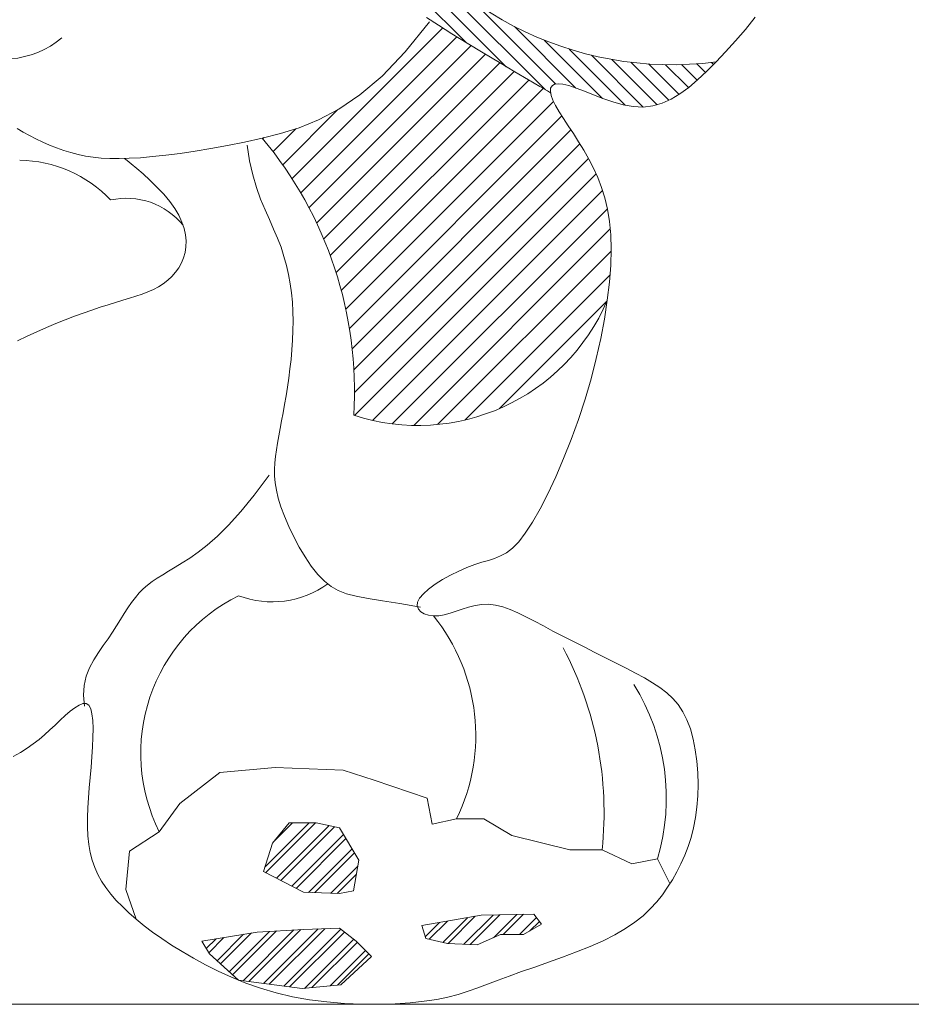
# Model space of a CAD drawing. Units: inches. Extents: x -17 to 1735, y -531 to 60.
# Tile 9 of 27: x 1734.675388 to 1734.679153, y -150.224179 to -150.220021. Entities that reach past the tile are written whole.
import ezdxf

# ---------------------------------------------------------------- set-up
doc = ezdxf.new("R2010")
doc.units = ezdxf.units.IN
doc.header["$MEASUREMENT"] = 0
doc.layers.add('A-FURN', color=242, linetype='Continuous', lineweight=18, true_color=0xcd2027)

# ---------------------------------------------------------------- blocks, each defined once
blk = doc.blocks.new('childrens_room_2')
for p, q in [((70.23120320653427, 54.05747840204134), (70.20236759360299, 54.08631401495807)), ((70.22698188498501, 54.05997091540342), (70.20319665329183, 54.0837561470675)), ((70.22263468104532, 54.06258931114138), (70.2050974529225, 54.08012653924237)), ((70.23229530256825, 54.0581151142091), (70.22340834805394, 54.06700206872341)), ((70.21842630278437, 54.06525539631406), (70.2196992340719, 54.06442092767832)), ((70.25366742467625, 54.06526988009722), (70.25262300519854, 54.06396623705081)), ((70.20400690125419, 54.04797145385822), (70.22016325000325, 54.06412780261456)), ((70.21614516905859, 54.06155212750167), (70.21875777329436, 54.06477708416645)), ((70.2196992340719, 54.06442092767832), (70.22114598193323, 54.06350699770559)), ((70.23445100571146, 54.05768821923851), (70.22784723080579, 54.06429199416601)), ((70.20494434069727, 54.04643916731441), (70.22168184573414, 54.06317667238039)), ((70.22114598193323, 54.06350699770559), (70.22277310794335, 54.06250397992557)), ((70.25262300519854, 54.06396623705081), (70.2515651093668, 54.06273375425229)), ((70.2058254618419, 54.04485056245033), (70.22321238294128, 54.06223748356428)), ((70.22277310794335, 54.06250397992557), (70.22450529499795, 54.06145310850701)), ((70.23729513219908, 54.05657290098173), (70.2310376150522, 54.06283041811406)), ((70.2515651093668, 54.06273375425229), (70.25051106391359, 54.06157435496282)), ((70.2066481458128, 54.04320352047074), (70.22475057818112, 54.06130595283906)), ((70.21366017778521, 54.05897447190222), (70.21614516905859, 54.06155212750167)), ((70.22450529499795, 54.06145310850701), (70.22624675651198, 54.06040833276205)), ((70.23974478501944, 54.05585205634128), (70.23372672202416, 54.06187011934384)), ((70.24167690089556, 54.05564874865962), (70.23611844704602, 54.06120720250914)), ((70.25051106391359, 54.06157435496282), (70.24947819562979, 54.06048996242901)), ((70.20740978735151, 54.04149543597163), (70.22629435937736, 54.06038000802658)), ((70.22624675651198, 54.06040833276205), (70.22790170590045, 54.05942360201009)), ((70.24315860012896, 54.0558958576425), (70.23830463429798, 54.06074982344438)), ((70.24441215903383, 54.05637110691754), (70.24033614836983, 54.06044711760336)), ((70.24551432266483, 54.05699775149554), (70.24224470166838, 54.06026737249925)), ((70.24651573046461, 54.05772515188295), (70.24405166280806, 54.06018921954677)), ((70.24745069189115, 54.05851899867997), (70.24577224395355, 54.06019744662484)), ((70.24834285863793, 54.05935564009855), (70.24741772615701, 54.06028077257946)), ((70.24947819562979, 54.06048996242901), (70.24847917870969, 54.05948426287654)), ((70.24920867151698, 54.0602186354285), (70.24899674283691, 54.06043056410857)), ((70.20810719999602, 54.03972312265108), (70.22784275591724, 54.05945867853592)), ((70.21129174275441, 54.05695870166386), (70.21366017778521, 54.05897447190222)), ((70.22790170590045, 54.05942360201009), (70.22937435646193, 54.05855286557784)), ((70.24847917870969, 54.05948426287654), (70.24750807719423, 54.05856799445468)), ((70.20873648953742, 54.03788268616921), (70.22939470015584, 54.05854089683129)), ((70.22937435646193, 54.05855286557784), (70.23056892155321, 54.05785007276285)), ((70.23056892155321, 54.05785007276285), (70.23138961453108, 54.05736917290636)), ((70.2318895930762, 54.05793588597447), (70.23174087157125, 54.05768089501947)), ((70.23215767678224, 54.05809471441756), (70.2318895930762, 54.05793588597447)), ((70.23254801054603, 54.05815257223588), (70.23215767678224, 54.05809471441756)), ((70.23306348210784, 54.05810465128019), (70.23254801054603, 54.05815257223588)), ((70.23370697932435, 54.0579461434449), (70.23306348210784, 54.05810465128019)), ((70.23447721871665, 54.05767913224412), (70.23370697932435, 54.0579461434449)), ((70.2465543024114, 54.05775365828453), (70.2456072658056, 54.05705375550173)), ((70.24750807719423, 54.05856799445468), (70.2465543024114, 54.05775365828453)), ((70.20902880730458, 54.05541940107508), (70.21129174275441, 54.05695870166386)), ((70.20929288009532, 54.03596935074023), (70.23095019063797, 54.05762666126832)), ((70.23138961453108, 54.05736917290636), (70.23174064886874, 54.05716411530597)), ((70.23174087157125, 54.05768089501947), (70.2317086245271, 54.05733454967998)), ((70.2317086245271, 54.05733454967998), (70.23178996414529, 54.05690165809068)), ((70.23178996414529, 54.05690165809068), (70.23198200256913, 54.05638702836444)), ((70.23535623175442, 54.05733326777994), (70.23447721871665, 54.05767913224412)), ((70.23632187868819, 54.05694509181052), (70.23535623175442, 54.05733326777994)), ((70.23735201976845, 54.05655114608674), (70.23632187868819, 54.05694509181052)), ((70.2456072658056, 54.05705375550173), (70.24465637882125, 54.05648078722737)), ((70.20977047372028, 54.0339772183492), (70.2320358858083, 54.05624263048088)), ((70.23198200256913, 54.05638702836444), (70.23227928510053, 54.05579578918554)), ((70.23227928510053, 54.05579578918554), (70.23266608932639, 54.05513435136384)), ((70.23842451512931, 54.05618797235951), (70.23735201976845, 54.05655114608674)), ((70.23951722507948, 54.05589211238697), (70.23842451512931, 54.05618797235951)), ((70.24060800981127, 54.05570010792001), (70.23951722507948, 54.05589211238697)), ((70.24167472957518, 54.05564850070954), (70.24060800981127, 54.05570010792001)), ((70.24270069931984, 54.05576565871019), (70.24167472957518, 54.05564850070954)), ((70.24369105284453, 54.05604725458982), (70.24270069931984, 54.05576565871019)), ((70.24465637882125, 54.05648078722737), (70.24369105284453, 54.05604725458982)), ((70.20301484620316, 54.04944912482318), (70.2089359568886, 54.05537023552319)), ((70.20686031459948, 54.05427115440983), (70.20902880730458, 54.05541940107508)), ((70.21016190813273, 54.03189892678205), (70.23294922768721, 54.05468624633653)), ((70.23266608932639, 54.05513435136384), (70.23312412575936, 54.05440944629521)), ((70.20477520797752, 54.05342854597114), (70.20686031459948, 54.05427115440983)), ((70.23312412575936, 54.05440944629521), (70.23363510520315, 54.05362780535364)), ((70.23363510520315, 54.05362780535364), (70.2341807381704, 54.05279615989861)), ((70.17451896065498, 54.0533605731602), (70.17516499910155, 54.05296905373546)), ((70.17516499910155, 54.05296905373546), (70.17584109301563, 54.05258956639449)), ((70.17584109301563, 54.05258956639449), (70.17654310266838, 54.05222553939387)), ((70.20081092616194, 54.05231858088376), (70.20276243071886, 54.05280616003295)), ((70.20196951501887, 54.05087351964761), (70.20441233455088, 54.05331633915051)), ((70.20276243071886, 54.05280616003295), (70.20477520797752, 54.05342854597114)), ((70.21045785759227, 54.02972515027653), (70.23392248806661, 54.05318978074359)), ((70.2341807381704, 54.05279615989861), (70.23474273529021, 54.05192124131867)), ((70.17654310266838, 54.05222553939387), (70.17726688838914, 54.05188040101205)), ((70.17726688838914, 54.05188040101205), (70.1780083105655, 54.05155757950564)), ((70.1780083105655, 54.05155757950564), (70.17876322946861, 54.0512605031385)), ((70.19530169218663, 54.05118995428932), (70.19707364461968, 54.05151860300105)), ((70.19707364461968, 54.05151860300105), (70.19891290449189, 54.0518944456839)), ((70.19891290449189, 54.0518944456839), (70.20081092616194, 54.05231858088376)), ((70.19944830472699, 54.04987592038963), (70.19918155060034, 54.051552788906)), ((70.20087192290114, 54.05224565353131), (70.20098945546081, 54.05236318604005)), ((70.21064627858462, 54.02744384521651), (70.23488772254089, 54.05168528922371)), ((70.23474273529021, 54.05192124131867), (70.23530280724982, 54.05100978098056)), ((70.17876322946861, 54.0512605031385), (70.17952750542784, 54.05099260018181)), ((70.17952750542784, 54.05099260018181), (70.18029699883076, 54.05075729889944)), ((70.18029699883076, 54.05075729889944), (70.18107070792351, 54.05055755143843)), ((70.18107070792351, 54.05055755143843), (70.18186018279405, 54.0503944055003)), ((70.18186018279405, 54.0503944055003), (70.18268011150533, 54.05026843268427)), ((70.18905787269935, 54.05032532816261), (70.19047513750732, 54.05047618649263)), ((70.19047513750732, 54.05047618649263), (70.19199389284361, 54.05066984459558)), ((70.19199389284361, 54.05066984459558), (70.1936055930087, 54.05090740101008)), ((70.1936055930087, 54.05090740101008), (70.19530169218663, 54.05118995428932)), ((70.23530280724982, 54.05100978098056), (70.23584266462015, 54.05006851025831)), ((70.18268011150533, 54.05026843268427), (70.1835451821203, 54.05018020457504)), ((70.1835451821203, 54.05018020457504), (70.18447008264368, 54.05013029277182)), ((70.18447008264368, 54.05013029277182), (70.18546950113844, 54.05011926885203)), ((70.18546950113844, 54.05011926885203), (70.18655812566752, 54.05014770441488)), ((70.18604057894439, 54.05013418576567), (70.1863111720991, 54.04991925461075)), ((70.1863111720991, 54.04991925461075), (70.18676120567719, 54.04955367698716)), ((70.18655812566752, 54.05014770441488), (70.18775064429386, 54.05021617104506)), ((70.18676120567719, 54.04955367698716), (70.18734889874352, 54.04906127812722)), ((70.18775064429386, 54.05021617104506), (70.18905787269935, 54.05032532816261)), ((70.1997931965266, 54.04836899507649), (70.19944830472699, 54.04987592038963)), ((70.21071122081369, 54.02503906145142), (70.23580548837666, 54.05013332902893)), ((70.23584266462015, 54.05006851025831), (70.2363459431904, 54.04910047430752)), ((70.18734889874352, 54.04906127812722), (70.18803247042118, 54.04846588327058)), ((70.18803247042118, 54.04846588327058), (70.18877013994964, 54.04779131765685)), ((70.20019748447115, 54.04700839372384), (70.1997931965266, 54.04836899507649)), ((70.21071357065696, 54.02257168532236), (70.23662629887579, 54.04848441356302)), ((70.2363459431904, 54.04910047430752), (70.23680397968158, 54.04809397335196)), ((70.18877013994964, 54.04779131765685), (70.18952012633557, 54.04706140653292)), ((70.23680397968158, 54.04809397335196), (70.23721003580025, 54.04703362138246)), ((70.18952012633557, 54.04706140653292), (70.19024064876024, 54.04629997513115)), ((70.19024064876024, 54.04629997513115), (70.19088992640494, 54.04553084869843)), ((70.2006424270908, 54.0457704971181), (70.20019748447115, 54.04700839372384)), ((70.21265150427237, 54.02203989292906), (70.2373123836692, 54.04670077231862)), ((70.23721003580025, 54.04703362138246), (70.23755737342756, 54.04590403241167)), ((70.19088992640494, 54.04553084869843), (70.19143405482058, 54.04477412162527)), ((70.20110928285752, 54.04463168603109), (70.2006424270908, 54.0457704971181)), ((70.23755737342756, 54.04590403241167), (70.23783925432829, 54.04468982043766)), ((70.19143405482058, 54.04477412162527), (70.19187063579332, 54.04403496495655)), ((70.19187063579332, 54.04403496495655), (70.1922051476536, 54.04331481888078)), ((70.20157931024326, 54.04356834124195), (70.20110928285752, 54.04463168603109)), ((70.2147521691036, 54.02167083178795), (70.23782642419567, 54.04474508685092)), ((70.23783925432829, 54.04468982043766), (70.2380489403836, 54.04337559945128)), ((70.1922051476536, 54.04331481888078), (70.19244306867361, 54.04261512360102)), ((70.20203376783641, 54.0425568435225), (70.20157931024326, 54.04356834124195)), ((70.2380489403836, 54.04337559945128), (70.23817969335826, 54.04194598346515)), ((70.19244306867361, 54.04261512360102), (70.19258987712558, 54.04193731929848)), ((70.19258987712558, 54.04193731929848), (70.19265105128173, 54.04128284617621)), ((70.2024539139343, 54.0415735736446), (70.20203376783641, 54.0425568435225)), ((70.21705303836964, 54.02150197504528), (70.23812249018695, 54.04257142684804)), ((70.23817969335826, 54.04194598346515), (70.23822477507522, 54.04038558647011)), ((70.19265105128173, 54.04128284617621), (70.19263206947247, 54.04065314442999)), ((70.2028244671051, 54.04059846488093), (70.2024539139343, 54.0415735736446)), ((70.19253840997001, 54.0400496542556), (70.1923754068662, 54.03947386384828)), ((70.19263206947247, 54.04065314442999), (70.19253840997001, 54.0400496542556)), ((70.20314398571966, 54.03962566042031), (70.2028244671051, 54.04059846488093)), ((70.2196183791489, 54.02159758981582), (70.23821973999614, 54.0401989506849)), ((70.23822477507522, 54.04038558647011), (70.23817889119849, 54.03868479222587)), ((70.1921478176478, 54.03892745344496), (70.19186025562115, 54.03841215128199)), ((70.1923754068662, 54.03947386384828), (70.1921478176478, 54.03892745344496)), ((70.20341448807042, 54.03865285595969), (70.20314398571966, 54.03962566042031)), ((70.19151733403444, 54.03792968558121), (70.19112366625225, 54.03748178460086)), ((70.19186025562115, 54.03841215128199), (70.19151733403444, 54.03792968558121)), ((70.20363799244981, 54.03767774718875), (70.20341448807042, 54.03865285595969)), ((70.23817889119849, 54.03868479222587), (70.2380425230472, 54.03685706347317)), ((70.19020254515229, 54.03669658970324), (70.18968431850547, 54.03636275226602)), ((70.19068386552274, 54.03707017656273), (70.19020254515229, 54.03669658970324)), ((70.19112366625225, 54.03748178460086), (70.19068386552274, 54.03707017656273)), ((70.20381651726669, 54.03669802978988), (70.20363799244981, 54.03767774718875)), ((70.20395208075527, 54.03571139945274), (70.20381651726669, 54.03669802978988)), ((70.22257581208717, 54.02208529677449), (70.23809855385801, 54.0376080385235)), ((70.2380425230472, 54.03685706347317), (70.23781759589795, 54.0349216327217)), ((70.18854791049264, 54.03580741270565), (70.18792838359835, 54.03557035645502)), ((70.18913283764735, 54.03606866425111), (70.18854791049264, 54.03580741270565)), ((70.18968431850547, 54.03636275226602), (70.18913283764735, 54.03606866425111)), ((70.2040467012662, 54.03471555186701), (70.20395208075527, 54.03571139945274)), ((70.18508121279186, 54.03469126083513), (70.18427138764994, 54.03444556337348)), ((70.18585067161942, 54.03491794768928), (70.18508121279186, 54.03469126083513)), ((70.18658091751743, 54.03513426512512), (70.18585067161942, 54.03491794768928)), ((70.18727310369607, 54.03534885432458), (70.18658091751743, 54.03513426512512)), ((70.18792838359835, 54.03557035645502), (70.18727310369607, 54.03534885432458)), ((70.20410239720835, 54.03370818271509), (70.2040467012662, 54.03471555186701)), ((70.22626748833457, 54.02330724702773), (70.2377693360427, 54.03480909471404)), ((70.23781759589795, 54.0349216327217), (70.23750603485271, 54.03289773246655)), ((70.18161153590657, 54.03354947326301), (70.18066071702518, 54.03319816138395)), ((70.18253294507625, 54.03387486160358), (70.18161153590657, 54.03354947326301)), ((70.18342090783293, 54.034173750339), (70.18253294507625, 54.03387486160358)), ((70.18427138764994, 54.03444556337348), (70.18342090783293, 54.034173750339)), ((70.20412142703893, 54.03268823586262), (70.20410239720835, 54.03370818271509)), ((70.17868699658314, 54.03242007136435), (70.17767216825044, 54.03199444538626)), ((70.17968452507515, 54.0328215020549), (70.17868699658314, 54.03242007136435)), ((70.18066071702518, 54.03319816138395), (70.17968452507515, 54.0328215020549)), ((70.20410701051472, 54.03165964784278), (70.20412142703893, 54.03268823586262)), ((70.23750603485271, 54.03289773246655), (70.23710976507166, 54.0308045952101)), ((70.17664407677833, 54.03154520020911), (70.17560685473612, 54.03107358400887)), ((70.17767216825044, 54.03199444538626), (70.17664407677833, 54.03154520020911)), ((70.2040626076155, 54.03062760335746), (70.20410701051472, 54.03165964784278)), ((70.17560685473612, 54.03107358400887), (70.17456501944574, 54.03058353331147)), ((70.20399167832105, 54.02959728711579), (70.2040626076155, 54.03062760335746)), ((70.23710976507166, 54.0308045952101), (70.2366307118896, 54.02866145344745)), ((70.20389768249473, 54.02857388381239), (70.20399167832105, 54.02959728711579)), ((70.20378408023274, 54.02756257816367), (70.20389768249473, 54.02857388381239)), ((70.2366307118896, 54.02866145344745), (70.2360708004085, 54.02648753968827)), ((70.20365433139843, 54.02656855487151), (70.20378408023274, 54.02756257816367)), ((70.20351189597162, 54.02559699863053), (70.20365433139843, 54.02656855487151)), ((70.2360708004085, 54.02648753968827), (70.23543195578851, 54.02430208643494)), ((70.20336023393205, 54.02465232605613), (70.20351189597162, 54.02559699863053)), ((70.2032028052595, 54.02373588132326), (70.20336023393205, 54.02465232605613)), ((70.23543195578851, 54.02430208643494), (70.23471867026413, 54.022126730239)), ((70.20304306993378, 54.02284824050588), (70.2032028052595, 54.02373588132326)), ((70.20273051918369, 54.02116167492789), (70.20288448787645, 54.02198997967793)), ((70.20288448787645, 54.02198997967793), (70.20304306993378, 54.02284824050588)), ((70.23471867026413, 54.022126730239), (70.23394570355188, 54.01999272392862)), ((70.20258462371888, 54.02036390232246), (70.20273051918369, 54.02116167492789)), ((70.20245026152, 54.01959723794283), (70.20258462371888, 54.02036390232246)), ((70.23394570355188, 54.01999272392862), (70.23313038255904, 54.0179337243739)), ((70.20223093784765, 54.01815675377878), (70.20233089256683, 54.01886225786296)), ((70.20233089256683, 54.01886225786296), (70.20245026152, 54.01959723794283)), ((70.2021586629667, 54.01746737988872), (70.20223093784765, 54.01815675377878)), ((70.23313038255904, 54.0179337243739), (70.23229003396003, 54.01598338845218)), ((70.2021232944203, 54.01677800598412), (70.2021586629667, 54.01746737988872)), ((70.20213405882126, 54.01607250187812), (70.2021232944203, 54.01677800598412)), ((70.20154355682783, 54.01615852959224), (70.1999571128504, 54.01402910353358)), ((70.20220018278226, 54.01533473737657), (70.20213405882126, 54.01607250187812)), ((70.23229003396003, 54.01598338845218), (70.23144198466208, 54.01417537304809)), ((70.20233089279967, 54.01454858228539), (70.20220018278226, 54.01533473737657)), ((70.20253541554442, 54.01369790641769), (70.20233089279967, 54.01454858228539)), ((70.1999571128504, 54.01402910353358), (70.19851223927574, 54.01225771024332)), ((70.20282297745464, 54.01276657957208), (70.20253541554442, 54.01369790641769)), ((70.23144198466208, 54.01417537304809), (70.23060356128147, 54.01254333503169)), ((70.20319939335926, 54.0117468727098), (70.20282297745464, 54.01276657957208)), ((70.23060356128147, 54.01254333503169), (70.2297920907254, 54.01112093128034)), ((70.19851223927574, 54.01225771024332), (70.19719826786196, 54.01080143188886)), ((70.20365683019511, 54.01066466134802), (70.20319939335926, 54.0117468727098)), ((70.19719826786196, 54.01080143188886), (70.19600453036722, 54.00961735061577)), ((70.20418404311523, 54.00955422214469), (70.20365683019511, 54.01066466134802)), ((70.2297920907254, 54.01112093128034), (70.22902489972651, 54.00994181867139)), ((70.19600453036722, 54.00961735061577), (70.19492035854958, 54.00866254856959)), ((70.20476978715627, 54.00844983177961), (70.20418404311523, 54.00955422214469)), ((70.22902489972651, 54.00994181867139), (70.2283135394787, 54.00902651187647)), ((70.19492035854958, 54.00866254856959), (70.19393508422537, 54.0078941079177)), ((70.20540281741299, 54.0073857669035), (70.20476978715627, 54.00844983177961)), ((70.22764645878809, 54.00834295672979), (70.22700633086382, 54.0078459568453)), ((70.2283135394787, 54.00902651187647), (70.22764645878809, 54.00834295672979)), ((70.19303803903634, 54.0072691107984), (70.19221855485696, 54.00674463937178)), ((70.19393508422537, 54.0078941079177), (70.19303803903634, 54.0072691107984)), ((70.20607188909663, 54.00639630419613), (70.20540281741299, 54.0073857669035)), ((70.22573762620917, 54.00723083736233), (70.22507439589711, 54.00702232500629)), ((70.22637582891505, 54.00749031585149), (70.22573762620917, 54.00723083736233)), ((70.22700633086382, 54.0078459568453), (70.22637582891505, 54.00749031585149)), ((70.19146682841122, 54.00628267245924), (70.19077651640285, 54.00586477554174)), ((70.19221855485696, 54.00674463937178), (70.19146682841122, 54.00628267245924)), ((70.20676575718565, 54.00551572031549), (70.20607188909663, 54.00639630419613)), ((70.22276993510198, 54.00626071799928), (70.2218939703994, 54.0058747858115)), ((70.22360354546575, 54.00657741317122), (70.22276993510198, 54.00626071799928)), ((70.22436881124625, 54.0068195824046), (70.22360354546575, 54.00657741317122)), ((70.22507439589711, 54.00702232500629), (70.22436881124625, 54.0068195824046)), ((70.18955822255114, 54.00510704034099), (70.18901928416338, 54.00474012637864)), ((70.19014214055963, 54.00547741078338), (70.18955822255114, 54.00510704034099)), ((70.19077651640285, 54.00586477554174), (70.19014214055963, 54.00547741078338)), ((70.20747317694943, 54.00477829193409), (70.20676575718565, 54.00551572031549)), ((70.22015359207172, 54.00495675443238), (70.2193584855518, 54.00445542723758)), ((70.2210103048815, 54.0054350026316), (70.22015359207172, 54.00495675443238)), ((70.2218939703994, 54.0058747858115), (70.2210103048815, 54.0054350026316)), ((70.18805443304475, 54.00396251648493), (70.18761756371126, 54.00352474488176)), ((70.18851984712413, 54.00436313103859), (70.18805443304475, 54.00396251648493)), ((70.18901928416338, 54.00474012637864), (70.18851984712413, 54.00436313103859)), ((70.20819366770914, 54.00420629407602), (70.20747317694943, 54.00477829193409)), ((70.20896980627325, 54.00377399522989), (70.20819366770914, 54.00420629407602)), ((70.21865963890335, 54.00394640703456), (70.21809170570808, 54.00344507981793)), ((70.2193584855518, 54.00445542723758), (70.21865963890335, 54.00394640703456)), ((70.1872033283685, 54.00303930279045), (70.18680408615504, 54.00250777441982)), ((70.18761756371126, 54.00352474488176), (70.1872033283685, 54.00303930279045)), ((70.20985493390938, 54.00344366225039), (70.20896980627325, 54.00377399522989)), ((70.21090239171056, 54.00317756199223), (70.20985493390938, 54.00344366225039)), ((70.21216552094441, 54.00293796131013), (70.21090239171056, 54.00317756199223)), ((70.21369766264573, 54.0026871270515), (70.21216552094441, 54.00293796131013)), ((70.21768933943125, 54.00296683160417), (70.21747772815753, 54.00252560594385)), ((70.21809170570808, 54.00344507981793), (70.21768933943125, 54.00296683160417)), ((70.18641176390113, 54.00193476841235), (70.18601828837885, 54.00132489338142)), ((70.18680408615504, 54.00250777441982), (70.18641176390113, 54.00193476841235)), ((70.21555215808215, 54.00238732607107), (70.21369766264573, 54.0026871270515)), ((70.21778234846307, 54.00200082521627), (70.21555215808215, 54.00238732607107)), ((70.21747772815753, 54.00252560594385), (70.21744419763446, 54.00212957664774)), ((70.21744419763446, 54.00212957664774), (70.21756660805434, 54.00178547510444)), ((70.21756660805434, 54.00178547510444), (70.21782281972585, 54.00150003268066)), ((70.22159829189653, 54.00156269820439), (70.22225847410621, 54.00178723761786)), ((70.22225847410621, 54.00178723761786), (70.22293790826691, 54.0020002375299)), ((70.22293790826691, 54.0020002375299), (70.22363563185675, 54.00217573407139)), ((70.22363563185675, 54.00217573407139), (70.22435068217922, 54.0022877633732)), ((70.22435068217922, 54.0022877633732), (70.22508209665423, 54.00231036155168)), ((70.22508209665423, 54.00231036155168), (70.22583003581852, 54.00222397556212)), ((70.22583003581852, 54.00222397556212), (70.2265991521522, 54.00203469570846)), ((70.2265991521522, 54.00203469570846), (70.22739522119403, 54.00175502309725)), ((70.18601828837885, 54.00132489338142), (70.18561558624381, 54.00068275794769)), ((70.21782281972585, 54.00150003268066), (70.21819069284132, 54.00127998075771)), ((70.21819069284132, 54.00127998075771), (70.21864808759302, 54.00113205071687)), ((70.21864808759302, 54.00113205071687), (70.21917286423152, 54.00106297392489)), ((70.21917286423152, 54.00106297392489), (70.21974288306549, 54.00107948177032)), ((70.21974288306549, 54.00107948177032), (70.22033953376697, 54.00118285640786)), ((70.22033953376697, 54.00118285640786), (70.22095832421795, 54.00135258318044)), ((70.22095832421795, 54.00135258318044), (70.22159829189653, 54.00156269820439)), ((70.22739522119403, 54.00175502309725), (70.22822401859915, 54.00139745887139)), ((70.22822401859915, 54.00139745887139), (70.22909131996451, 54.00097450413745)), ((70.22909131996451, 54.00097450413745), (70.23000290082885, 54.00049866003104)), ((70.18519558420988, 54.00001297075363), (70.1847502091073, 53.99932014041991)), ((70.18561558624381, 54.00068275794769), (70.18519558420988, 54.00001297075363)), ((70.23000290082885, 54.00049866003104), (70.23096453684732, 53.99998242766599)), ((70.23096453684732, 53.99998242766599), (70.23198200350046, 53.99943830817796)), ((70.18427138764994, 53.99860887556719), (70.18375787035214, 53.9978810004381)), ((70.1847502091073, 53.99932014041991), (70.18427138764994, 53.99860887556719)), ((70.23198200350046, 53.99943830817796), (70.23305722606486, 53.99887752051876)), ((70.23305722606486, 53.99887752051876), (70.23417672818644, 53.99830615498507)), ((70.18375787035214, 53.9978810004381), (70.18323570316309, 53.99712720178508)), ((70.23417672818644, 53.99830615498507), (70.23532318295796, 53.99772901968976)), ((70.23532318295796, 53.99772901968976), (70.23647926376319, 53.99715092276022)), ((70.18323570316309, 53.99712720178508), (70.1827377558325, 53.99633538195343)), ((70.23647926376319, 53.99715092276022), (70.23762764375309, 53.99657667232389)), ((70.23762764375309, 53.99657667232389), (70.23875099625323, 53.99601107650818)), ((70.18229689793546, 53.99549344331029), (70.18194599927986, 53.99458928820826)), ((70.1827377558325, 53.99633538195343), (70.18229689793546, 53.99549344331029)), ((70.23875099625323, 53.99601107650818), (70.23983199435636, 53.99545894343322)), ((70.23983199435636, 53.99545894343322), (70.24085331138807, 53.99492508121915)), ((70.18194599927986, 53.99458928820826), (70.18171792961542, 53.99361081901446)), ((70.24085331138807, 53.99492508121915), (70.24180066871807, 53.99441045150019)), ((70.24180066871807, 53.99441045150019), (70.2426719808241, 53.99390062989408)), ((70.18171792961542, 53.99361081901446), (70.18164555857541, 53.99254593807421)), ((70.2426719808241, 53.99390062989408), (70.24346821028624, 53.9933773455254)), ((70.24346821028624, 53.9933773455254), (70.24419031962636, 53.99282232753325)), ((70.18164555857541, 53.99254593807421), (70.18176175590955, 53.99138254775465)), ((70.24419031962636, 53.99282232753325), (70.244839271541, 53.9922173050349)), ((70.18116161007084, 53.99149592623001), (70.1807050173625, 53.99121192631577)), ((70.18157007278526, 53.99165299162127), (70.18116161007084, 53.99149592623001)), ((70.18192077964662, 53.99165619699346), (70.18157007278526, 53.99165299162127)), ((70.18220410450479, 53.99147861685055), (70.18192077964662, 53.99165619699346)), ((70.18241346966127, 53.99110214057731), (70.18220410450479, 53.99147861685055)), ((70.244839271541, 53.9922173050349), (70.24541602849379, 53.99154400715492)), ((70.24541602849379, 53.99154400715492), (70.24592155323947, 53.99078416302512)), ((70.17968594609877, 53.9903708249389), (70.17914271955262, 53.98986757447568)), ((70.1802099207521, 53.99082791738186), (70.17968594609877, 53.9903708249389)), ((70.1807050173625, 53.99121192631577), (70.1802099207521, 53.99082791738186)), ((70.1825544903509, 53.9905439171693), (70.18241346966127, 53.99110214057731)), ((70.18263582985267, 53.98982991049564), (70.1825544903509, 53.9905439171693)), ((70.24592155323947, 53.99078416302512), (70.2463568082417, 53.98991950177009)), ((70.17858986703098, 53.98934509149552), (70.17803364544991, 53.98882613445898)), ((70.17914271955262, 53.98986757447568), (70.17858986703098, 53.98934509149552)), ((70.18266615167843, 53.98898608444), (70.18263582985267, 53.98982991049564)), ((70.2463568082417, 53.98991950177009), (70.24672275619699, 53.98893864416317)), ((70.17746683531325, 53.98831679366271), (70.17687884800719, 53.98781899236059)), ((70.17803364544991, 53.98882613445898), (70.17746683531325, 53.98831679366271)), ((70.18265411910718, 53.98803840287877), (70.18266615167843, 53.98898608444)), ((70.24672275619699, 53.98893864416317), (70.24702035962721, 53.98785777755114)), ((70.17625909497613, 53.9873346538065), (70.17559698760627, 53.98686570126159)), ((70.17687884800719, 53.98781899236059), (70.17625909497613, 53.9873346538065)), ((70.18253764458817, 53.98593532877424), (70.18260839559255, 53.9870128297029)), ((70.18260839559255, 53.9870128297029), (70.18265411910718, 53.98803840287877)), ((70.24702035962721, 53.98785777755114), (70.24725058117068, 53.98669998094414)), ((70.17488193734201, 53.98641405797246), (70.17410335556954, 53.985981647193)), ((70.17559698760627, 53.98686570126159), (70.17488193734201, 53.98641405797246)), ((70.18245052937301, 53.98483186399102), (70.18253764458817, 53.98593532877424)), ((70.24725058117068, 53.98669998094414), (70.24741438340746, 53.98548833333774)), ((70.24741438340746, 53.98548833333774), (70.24751272891766, 53.98424591373481)), ((70.18235571345897, 53.98372519380649), (70.18245052937301, 53.98483186399102)), ((70.19625148678782, 53.98425861792787), (70.19197089150433, 53.98094796042136)), ((70.20218908805285, 53.98481039490292), (70.19625148678782, 53.98425861792787)), ((70.2095075273642, 53.98453450696109), (70.20218908805285, 53.98481039490292)), ((70.21282153560199, 53.98343095409512), (70.2095075273642, 53.98453450696109)), ((70.24751272891766, 53.98424591373481), (70.24754658039777, 53.98299580112364)), ((70.1822618601832, 53.98262525501053), (70.18235571345897, 53.98372519380649)), ((70.21848296887359, 53.98149973631229), (70.21282153560199, 53.98343095409512)), ((70.24754658039777, 53.98299580112364), (70.24751690031147, 53.98176107452167)), ((70.18217763288297, 53.98153877896987), (70.1822618601832, 53.98262525501053)), ((70.24751690031147, 53.98176107452167), (70.24742465135526, 53.98056481291718)), ((70.18211169495365, 53.98047249707309), (70.18217763288297, 53.98153877896987)), ((70.19197089150433, 53.98094796042136), (70.18976155145677, 53.97791318977255)), ((70.21903530486045, 53.97874085468941), (70.21848296887359, 53.98149973631229)), ((70.18207270984888, 53.97943314067965), (70.18211169495365, 53.98047249707309)), ((70.24742465135526, 53.98056481291718), (70.24727127737017, 53.97942544745314)), ((70.18206934084768, 53.97842744116355), (70.18207270984888, 53.97943314067965)), ((70.20111043187674, 53.97415213506469), (70.2058370959817, 53.97887879920602)), ((70.20117600478582, 53.97351850347916), (70.20653630049085, 53.97887879920602)), ((70.20191292005941, 53.97667169348136), (70.20370800910635, 53.97887879920602)), ((70.20214579854976, 53.97695802328093), (70.20406657446759, 53.97887879920602)), ((70.20234419779038, 53.97291617502782), (70.2079981585953, 53.97857013580363)), ((70.20370800910635, 53.97887879920602), (70.20660776826438, 53.97887879920602)), ((70.20660776826438, 53.97887879920602), (70.20909327636357, 53.97832702223098)), ((70.22165889602503, 53.97929263058035), (70.21903530486045, 53.97874085468941)), ((70.22455865512487, 53.97929263058035), (70.22165889602503, 53.97929263058035)), ((70.22759649729008, 53.97749935730684), (70.22455865512487, 53.97929263058035)), ((70.24727127737017, 53.97942544745314), (70.24706014747383, 53.97834281786931)), ((70.18211025140366, 53.97746212990608), (70.18206934084768, 53.97842744116355)), ((70.18976155145677, 53.97791318977255), (70.18658562622616, 53.97584402855722)), ((70.20280553413207, 53.97267830683126), (70.20857034013491, 53.97844311284865)), ((70.20397372719484, 53.9720759783799), (70.20951785509126, 53.97762010631999)), ((70.20909327636357, 53.97832702223098), (70.21116453148309, 53.97487842020786)), ((70.23381026462769, 53.97598197307383), (70.22759649729008, 53.97749935730684)), ((70.24706014747383, 53.97834281786931), (70.2467951120448, 53.97731211603098)), ((70.18220410485404, 53.97654393826673), (70.18211025140366, 53.97746212990608)), ((70.18235812063679, 53.97567735383785), (70.18220410485404, 53.97654393826673)), ((70.20094633499278, 53.97363692283255), (70.20191292005941, 53.97667169348136)), ((70.20443506347831, 53.97183811018334), (70.20978022257216, 53.97718326929174)), ((70.2467951120448, 53.97731211603098), (70.24648002146162, 53.97632853382532)), ((70.18257374276757, 53.97485788902708), (70.18235812063679, 53.97567735383785)), ((70.18658562622616, 53.97584402855722), (70.18617137522554, 53.97170570613383)), ((70.20577764442307, 53.97141016965765), (70.21044458793361, 53.97607711312452)), ((70.20645276190363, 53.97138608264362), (70.2107069553563, 53.97564027609627)), ((70.23726235785173, 53.97598197307383), (70.23381026462769, 53.97598197307383)), ((70.24043828494499, 53.97446458774942), (70.23726235785173, 53.97598197307383)), ((70.24611872610288, 53.9753872631249), (70.24571507646354, 53.97448349579502)), ((70.24648002146162, 53.97632853382532), (70.24611872610288, 53.9753872631249)), ((70.18285097118817, 53.97407881246039), (70.18257374276757, 53.97485788902708)), ((70.21116453148309, 53.97487842020786), (70.21061219741706, 53.97156776161722)), ((70.24319995911677, 53.97501636364035), (70.24043828494499, 53.97446458774942)), ((70.24454078638112, 53.97235958649111), (70.24319995911677, 53.97501636364035)), ((70.24571507646354, 53.97448349579502), (70.24527292286396, 53.97361242372284)), ((70.18318980584039, 53.97333339276378), (70.18285097118817, 53.97407881246039)), ((70.18359024684062, 53.97261489854867), (70.18318980584039, 53.97333339276378)), ((70.20522693021806, 53.97142981818473), (70.20094633499278, 53.97363692283255)), ((70.20816229040386, 53.97132508962972), (70.21105417988613, 53.97421697910471)), ((70.20883740788443, 53.97130100261569), (70.21091416939046, 53.97337776409989)), ((70.24527292286396, 53.97361242372284), (70.2447961156827, 53.97276923878092)), ((70.18405229413068, 53.9719165984556), (70.18359024684062, 53.97261489854867)), ((70.2447961156827, 53.97276923878092), (70.24428545707954, 53.97194993420129)), ((70.18457594776876, 53.97123176109602), (70.18405229413068, 53.9719165984556)), ((70.18516120763846, 53.9705536550959), (70.18457594776876, 53.97123176109602)), ((70.18617137522554, 53.97170570613383), (70.18729528867291, 53.96851837538855)), ((70.20909327636357, 53.97129187366812), (70.20522693021806, 53.97142981818473)), ((70.21061219741706, 53.97156776161722), (70.20909327636357, 53.97129187366812)), ((70.2437295563391, 53.97115370862451), (70.24311397452723, 53.97038056205059)), ((70.24428545707954, 53.97194993420129), (70.2437295563391, 53.97115370862451)), ((70.18580839475501, 53.96987651070816), (70.18516120763846, 53.9705536550959)), ((70.24311397452723, 53.97038056205059), (70.24242427259335, 53.96963049449408)), ((70.18651911332157, 53.96919840467893), (70.18580839475501, 53.96987651070816)), ((70.18729528867291, 53.96851837538855), (70.18651911332157, 53.96919840467893)), ((70.22994392040303, 53.96908476794346), (70.22428248713143, 53.96894682451097)), ((70.22561391892262, 53.96654918418647), (70.22810468899436, 53.96903995422184)), ((70.2266416014277, 53.96687766221152), (70.22882135539433, 53.96905741612721)), ((70.23077242246248, 53.96798121507749), (70.22994392040303, 53.96908476794346)), ((70.24242427259335, 53.96963049449408), (70.24164601160331, 53.96890350593316)), ((70.18813884585282, 53.96783546122463), (70.18729528867291, 53.96851837538855)), ((70.22428248713143, 53.96894682451097), (70.21793063480757, 53.967843271645)), ((70.21829280729756, 53.96663725052935), (70.2198285703885, 53.96817301360574)), ((70.21872843610939, 53.96637367486841), (70.22067479563296, 53.96832003439198)), ((70.22016199126259, 53.96603670847838), (70.22281760234503, 53.9686923195681)), ((70.22073469987257, 53.96591021263742), (70.22366382758949, 53.96883934035435)), ((70.22243152100012, 53.96583651222176), (70.22557328415454, 53.96897827537618)), ((70.2231016201072, 53.96580740685607), (70.2262899505545, 53.96899573728155)), ((70.2284121229418, 53.96687766221152), (70.23023350549514, 53.96869904475756)), ((70.22883925035015, 53.96687766221152), (70.23077242246248, 53.96798121507749)), ((70.22947324219741, 53.96723957696526), (70.2305333377549, 53.96829967250818)), ((70.24076475256473, 53.96819959638236), (70.23976605654346, 53.9675187658417)), ((70.24164601160331, 53.96890350593316), (70.24076475256473, 53.96819959638236)), ((70.18905171019608, 53.96714870055297), (70.18813884585282, 53.96783546122463)), ((70.19003580680467, 53.96645713176844), (70.18905171019608, 53.96714870055297)), ((70.19431831467548, 53.96618794181126), (70.20025591594052, 53.96715355124474)), ((70.19633598970134, 53.96373903642092), (70.1996523486555, 53.9670553954042)), ((70.19726816950018, 53.96290069472019), (70.2015953644982, 53.96722788974006)), ((70.19763630076662, 53.96256962149204), (70.20233565459378, 53.96726897534103)), ((70.19876223140048, 53.96192503059722), (70.20421021281393, 53.96737301206162)), ((70.19937939419063, 53.96184298894372), (70.2049505029677, 53.96741409766258)), ((70.20025591594052, 53.96715355124474), (70.20522693021806, 53.96742943918656)), ((70.20094217035106, 53.96163524355364), (70.20679221210187, 53.96748528528991)), ((70.2015593331412, 53.96155320190013), (70.20751728572534, 53.96751115444789)), ((70.20312210930163, 53.96134545650278), (70.20923507203, 53.9674584192457)), ((70.20373927209178, 53.96126341484927), (70.20963044826524, 53.96715459101546)), ((70.20522693021806, 53.96742943918656), (70.20909327636357, 53.96756738261905)), ((70.20909327636357, 53.96756738261905), (70.21088836348964, 53.96618794181126)), ((70.21793063480757, 53.967843271645), (70.2183448858664, 53.96646383083719)), ((70.23976605654346, 53.9675187658417), (70.23863548448892, 53.96686101429662)), ((70.19109306089697, 53.96575979322955), (70.19003580680467, 53.96645713176844)), ((70.19514681673493, 53.96480850099618), (70.19431831467548, 53.96618794181126)), ((70.19480524108397, 53.96537721825592), (70.19586798089907, 53.96643995811468)), ((70.19506760850666, 53.96494038122767), (70.19670297776932, 53.96657575046851)), ((70.19596785843488, 53.96407010964907), (70.19881735184347, 53.96691960305765)), ((70.20535719774082, 53.96111081896236), (70.21063161770465, 53.96638523895529)), ((70.20613400435425, 53.96118842109576), (70.21101100633271, 53.96606542308877)), ((70.21088836348964, 53.96618794181126), (70.21254536952941, 53.96453261305436)), ((70.2183448858664, 53.96646383083719), (70.22069230897935, 53.96591205386215)), ((70.22069230897935, 53.96591205386215), (70.2238682360726, 53.96577410934554)), ((70.2238682360726, 53.96577410934554), (70.22635374230914, 53.96687766221152)), ((70.22635374230914, 53.96687766221152), (70.22883925035015, 53.96687766221152)), ((70.23736677960144, 53.96622634176896), (70.23598641327001, 53.96561474823688)), ((70.23863548448892, 53.96686101429662), (70.23736677960144, 53.96622634176896)), ((70.19222539774958, 53.9650557233312), (70.19109306089697, 53.96575979322955)), ((70.19343442156563, 53.96434620424265), (70.19222539774958, 53.9650557233312)), ((70.2081010295183, 53.96138492477479), (70.21189671540517, 53.96518061061073)), ((70.20887783618994, 53.96146252690818), (70.21224649466924, 53.96483118539475)), ((70.2345290390763, 53.96502623370764), (70.2330293105438, 53.96446079818128)), ((70.23598641327001, 53.96561474823688), (70.2345290390763, 53.96502623370764)), ((70.19472045336036, 53.96364149328878), (70.19343442156563, 53.96434620424265)), ((70.19828206819832, 53.96198886040514), (70.19514681673493, 53.96480850099618)), ((70.21254536952941, 53.96453261305436), (70.20923135937076, 53.96149784348967)), ((70.23152188119595, 53.96391844165049), (70.23004140461447, 53.96339916411529)), ((70.2330293105438, 53.96446079818128), (70.23152188119595, 53.96391844165049)), ((70.19608349295916, 53.96295409159796), (70.19472045336036, 53.96364149328878)), ((70.19752354047844, 53.96229650029858), (70.19608349295916, 53.96295409159796)), ((70.2286225343228, 53.96290296557566), (70.22729992390262, 53.96242984602435)), ((70.23004140461447, 53.96339916411529), (70.2286225343228, 53.96290296557566)), ((70.1990405959182, 53.96168122050443), (70.19752354047844, 53.96229650029858)), ((70.20508884715267, 53.96108401103123), (70.19828206819832, 53.96198886040514)), ((70.20063465916203, 53.96112075335117), (70.1990405959182, 53.96168122050443)), ((70.22609619436437, 53.96198028627845), (70.22498583678274, 53.96155669040166)), ((70.22729992390262, 53.96242984602435), (70.22609619436437, 53.96198028627845)), ((70.20230573032634, 53.9606275999526), (70.20063465916203, 53.96112075335117)), ((70.20405380941114, 53.9602142614371), (70.20230573032634, 53.9606275999526)), ((70.20923135937076, 53.96149784348967), (70.20508884715267, 53.96108401103123)), ((70.22289507249253, 53.96079892974961), (70.2218395830819, 53.96047053474325)), ((70.22393131001039, 53.96116194326754), (70.22289507249253, 53.96079892974961)), ((70.22498583678274, 53.96155669040166), (70.22393131001039, 53.96116194326754)), ((70.2058737624425, 53.9598901937847), (70.20405380941114, 53.9602142614371)), ((70.20773992019124, 53.95965267239666), (70.2058737624425, 53.9598901937847)), ((70.20962147951244, 53.95949592751134), (70.20773992019124, 53.95965267239666)), ((70.21668566962356, 53.95956131807037), (70.21505053546164, 53.95945265441554)), ((70.21818218951697, 53.95972190949255), (70.21668566962356, 53.95956131807037)), ((70.21952068294516, 53.95992913973026), (70.21818218951697, 53.95972190949255)), ((70.22072730034007, 53.96017964310743), (70.21952068294516, 53.95992913973026)), ((70.2218395830819, 53.96047053474325), (70.22072730034007, 53.96017964310743)), ((69.75691338651995, 53.95940168826786), (71.77791338646966, 53.95940168826786)), ((70.21148763726117, 53.95941418938895), (70.20962147951244, 53.95949592751134)), ((70.21330759029254, 53.95940168826786), (70.21148763726117, 53.95941418938895)), ((70.21505053546164, 53.95945265441554), (70.21330759029254, 53.95940168826786))]:
    blk.add_line(p, q)
for centre, radius, start, end in [((70.2447362221533, 54.09694509747208), 0.0367622521574525, 207.5719883014331, 277.4112487822124), ((70.17302459694795, 54.07056868865623), 0.0097912997460796, 239.7089148198155, 310.1368033599684), ((70.16834037955735, 54.02509808719918), 0.0423708823452092, 356.6153251743423, 39.97355406391458), ((70.17465436372325, 54.03632152119683), 0.0136224427040684, 43.39816713550395, 89.38562918617615), ((70.18624259998208, 54.03804034062199), 0.007825390013488, 38.99955824035533, 102.473682377326), ((70.21751530137729, 54.04356128166404), 0.0220641495527858, 251.8367770201434, 336.9478037959915), ((70.20188800770441, 54.0127324692134), 0.0101611248879515, 249.1900331100195, 305.811031420364), ((70.20665663935827, 53.98632341033811), 0.0188726205627017, 116.3564178108619, 206.463702741566), ((70.20332153037774, 53.98822573859655), 0.0203975340880889, 334.0268190681756, 39.00235379868047), ((70.19963639696246, 53.97997639259705), 0.0378373930908262, 353.9401051043006, 27.82577847723737), ((70.22121168627521, 53.98155428536705), 0.0229396722355832, 343.440851376884, 31.98698738530506)]:
    blk.add_arc(centre, radius, start, end)

msp = doc.modelspace()

# ---------------------------------------------------------------- block references
at = {"layer": 'A-FURN', "xscale": 0.0393700787401575, "yscale": 0.0393700787401575, "zscale": 0.0393700787401575}
msp.add_blockref('childrens_room_2', (1731.912600860487, -152.3485650223338), dxfattribs=at)

doc.saveas('drawing.dxf')
